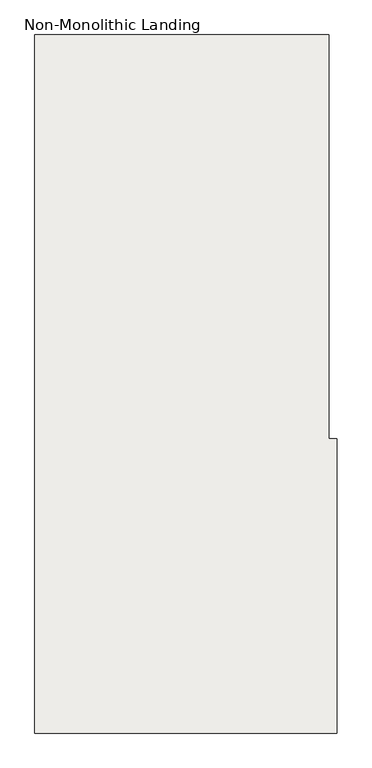
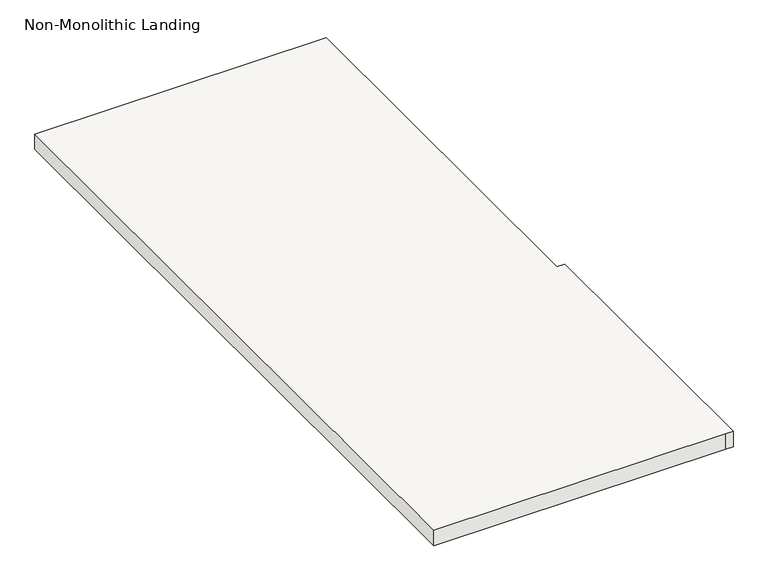
"""IFC4 building model written with IfcOpenShell, lengths in millimetres: slab geometry, Non-Monolithic Landing."""

from ifc_helpers import new_model, si_unit, origin, place, context, project, spatial, faceted_brep, source, transform, mapped, element, save


def non_monolithic_landing_6eacb0e7(model_context):
    return source(origin(), model_context, "Body", "Brep", [
        faceted_brep([(-12083.8120641, -2647.9669819, 5543.55), (-12058.4120641, -2647.9669819, 5568.95), (-12058.4120641, -3562.3669819, 5568.95), (-12083.8120641, -3562.3669819, 5543.55), (-12972.8120641, -2647.9669819, 5588.0), (-12972.8120641, -4817.9038196, 5588.0), (-12058.4120641, -4817.9038196, 5588.0), (-12033.0120641, -4817.9038196, 5588.0), (-12033.0120641, -3903.5038196, 5588.0), (-12058.4120641, -3903.5038196, 5588.0), (-12058.4120641, -2647.9669819, 5588.0), (-12083.8120641, -3562.3669819, 5537.2), (-12058.4120641, -3562.3669819, 5537.2), (-12058.4120641, -3903.5038196, 5537.2), (-12033.0120641, -3903.5038196, 5537.2), (-12033.0120641, -4817.9038196, 5537.2), (-12058.4120641, -4817.9038196, 5537.2), (-12972.8120641, -4817.9038196, 5537.2), (-12972.8120641, -2647.9669819, 5537.2), (-12083.8120641, -2647.9669819, 5537.2)], [[[0, 1, 2, 3]], [[4, 5, 6, 7, 8, 9, 10]], [[11, 12, 13, 14, 15, 16, 17, 18, 19]], [[12, 11, 3, 2]], [[11, 19, 0, 3]], [[4, 10, 1, 0, 19, 18]], [[5, 4, 18, 17]], [[6, 5, 17, 16]], [[7, 6, 16, 15]], [[8, 7, 15, 14]], [[9, 8, 14, 13]], [[10, 9, 13, 12, 2, 1]]]),
    ])


if __name__ == "__main__":
    model = new_model("IFC4")
    model_context = context("Model", 3, world=origin())
    ifc_project = project(units=[si_unit("LENGTHUNIT", "METRE", prefix="MILLI")], contexts=[model_context])
    site = spatial("IfcSite", under=ifc_project)
    building = spatial("IfcBuilding", under=site)
    placement = place(None, origin())
    non_monolithic_landing_shape = non_monolithic_landing_6eacb0e7(model_context)
    element("IfcSlab", 1, ObjectType="Non-Monolithic Landing", at=placement, inside=building, context=model_context, shape_type="MappedRepresentation", body=[
        mapped(non_monolithic_landing_shape, transform((0.0, 0.0, 0.0), x_axis=(1.0, 0.0, 0.0), y_axis=(0.0, 1.0, 0.0), z_axis=(0.0, 0.0, 1.0))),
    ])
    save(model, "model.ifc")
